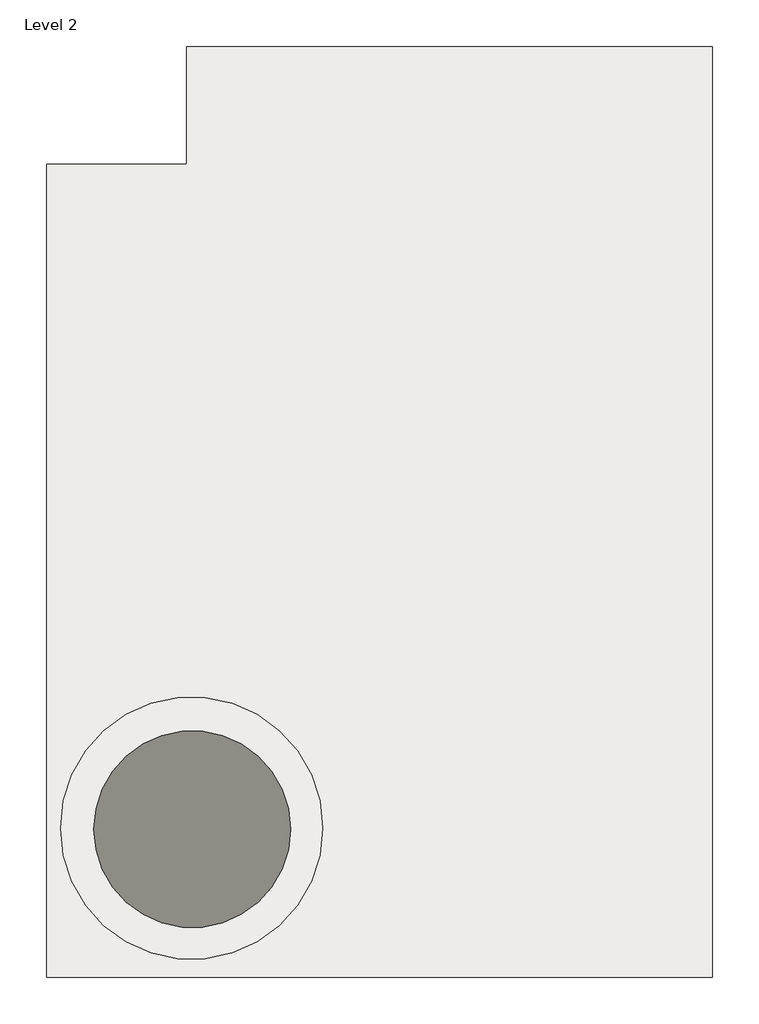
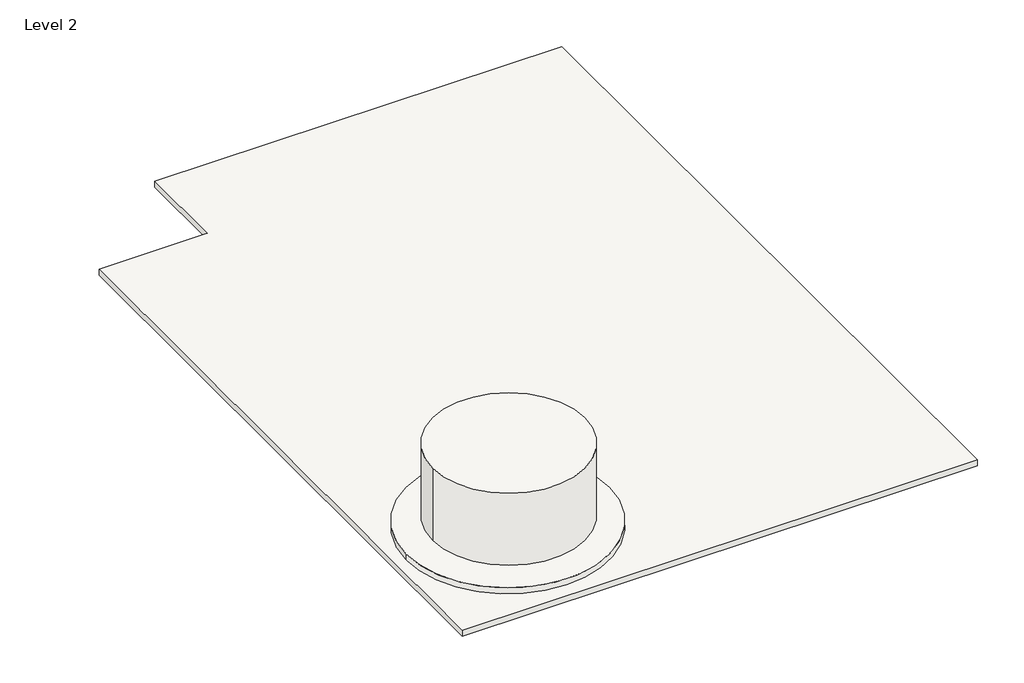
# One storey, incomplete: 3 slabs.
"""IFC4 building model written with IfcOpenShell, lengths in millimetres."""

from ifc_helpers import new_model, si_unit, point, frame, frame_2d, origin, place, context, project, spatial, polyline, circle_curve, trimmed, segment, composite_curve, outline, extrude, element, save

model = new_model("IFC4")

# Units and contexts
model_context = context("Model", 3, world=origin())
ifc_project = project(units=[si_unit("LENGTHUNIT", "METRE", prefix="MILLI")], contexts=[model_context])

# Site, building, storey
site = spatial("IfcSite", under=ifc_project)
building = spatial("IfcBuilding", under=site)
storey = spatial("IfcBuildingStorey", under=building, Name="Level 2", Elevation=3200.4)

# Slabs
placement = place(None, origin())
element("IfcSlab", 1, at=placement, inside=storey, context=model_context, shape_type="SweptSolid", body=[
    extrude(outline(polyline([(9606.3713581, 5669.0664065), (9606.3713581, 20788.4164065), (12209.8713581, 20788.4164065), (12209.8713581, 22972.8164065), (21988.8713581, 22972.8164065), (21988.8713581, 5669.0664065), (9606.3713581, 5669.0664065)])), frame((0.0, 0.0, 3048.0), z_axis=(0.0, 0.0, 1.0), x_axis=(1.0, 0.0, 0.0)), (0.0, 0.0, 1.0), 152.4),
])
element("IfcSlab", 2, at=placement, inside=storey, context=model_context, shape_type="SweptSolid", body=[
    extrude(outline(composite_curve([segment(trimmed(circle_curve(frame_2d((12304.3985738, 8446.0471671)), 2438.4), [point((9865.9985738, 8446.0471671))], [point((14742.7985738, 8446.0471671))], False, "CARTESIAN"), True, "CONTINUOUS"), segment(trimmed(circle_curve(frame_2d((12304.3985738, 8446.0471671)), 2438.4), [point((14742.7985738, 8446.0471671))], [point((9865.9985738, 8446.0471671))], False, "CARTESIAN"), True, "CONTINUOUS")], self_intersect=False)), frame((0.0, 0.0, 3200.4), z_axis=(0.0, 0.0, 1.0), x_axis=(1.0, 0.0, 0.0)), (0.0, 0.0, 1.0), 152.4),
])
element("IfcSlab", 3, at=placement, inside=storey, context=model_context, shape_type="SweptSolid", body=[
    extrude(outline(composite_curve([segment(trimmed(circle_curve(frame_2d((12315.55312, 8424.9664065)), 1828.8), [point((10486.75312, 8424.9664065))], [point((14144.35312, 8424.9664065))], False, "CARTESIAN"), True, "CONTINUOUS"), segment(trimmed(circle_curve(frame_2d((12315.55312, 8424.9664065)), 1828.8), [point((14144.35312, 8424.9664065))], [point((10486.75312, 8424.9664065))], False, "CARTESIAN"), True, "CONTINUOUS")], self_intersect=False)), frame((0.0, 0.0, 3505.2), z_axis=(0.0, 0.0, 1.0), x_axis=(1.0, 0.0, 0.0)), (0.0, 0.0, 1.0), 1828.8),
])

save(model, "model.ifc")

# Revit data of these elements
# Type
#   Assembly Code = "B1010"
#   Function = 0
#   Layers, outside or top first: 0' - 6" "Concrete, Cast-in-Place gray" (function 1)
# Type
#   Assembly Code = "B1010"
#   Function = 0
#   Layers, outside or top first: 6' - 0" "Concrete, Cast-in-Place gray" (function 1)
# Element 1 (IfcSlab)
#   built-in parameter 1001955 = -1.5708 (stored number, unit not read)
#   Height Offset From Level = 0' - 0"
#   Phase Created = New Construction
#   Materials on its faces: "Concrete, Cast-in-Place gray"
# Element 2 (IfcSlab)
#   Height Offset From Level = 0' - 6"
#   Phase Created = New Construction
#   Materials on its faces: "Concrete, Cast-in-Place gray"
# Element 3 (IfcSlab)
#   Height Offset From Level = 7' - 0"
#   Phase Created = New Construction
#   Materials on its faces: "Water", "Concrete, Cast-in-Place gray"
# Materials
#   "Concrete, Cast-in-Place gray": class "Concrete", colour RGB 192 192 192, transparency 0, Description = "Cast-in-place concrete", Cost = 0
#   "Water": class "Liquid", colour RGB 108 195 217, transparency 0.7, Description = "Water", Cost = 0
